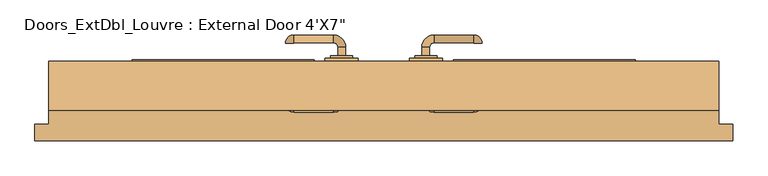
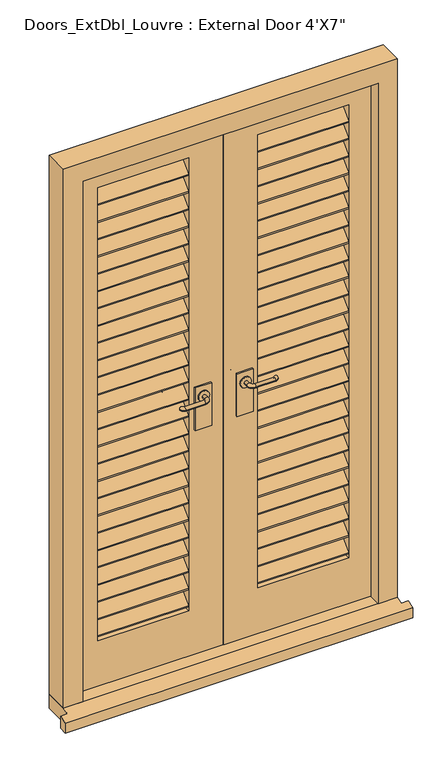
"""IFC4 building model written with IfcOpenShell, lengths in millimetres: door geometry."""

from ifc_helpers import new_model, si_unit, point, frame, frame_2d, origin, place, context, project, spatial, polyline, circle_curve, ellipse_curve, trimmed, segment, composite_curve, outline, extrude, faceted_brep, source, transform, mapped, element, save
from ifc_brep_helpers import plane_surface, cylinder_surface, revolved_surface, advanced_brep


def door_6c7b9bf3(model_context):
    return source(origin(), model_context, "Body", "SolidModel", [
        extrude(outline(polyline([(-0.3, 1896.068), (-0.3, 1900.468), (2.7, 1900.468), (2.7, 1894.8253593), (-41.3, 1850.8253593), (-41.3, 1847.668), (-44.3, 1847.668), (-44.3, 1852.068), (-0.3, 1896.068)])), frame((126.5, 0.0, 0.0), z_axis=(1.0, 0.0, 0.0), x_axis=(0.0, 1.0, 0.0)), (0.0, 0.0, 1.0), 331.6),
        extrude(outline(polyline([(-0.3, 1829.436), (-0.3, 1833.836), (2.7, 1833.836), (2.7, 1828.1933593), (-41.3, 1784.1933593), (-41.3, 1781.036), (-44.3, 1781.036), (-44.3, 1785.436), (-0.3, 1829.436)])), frame((126.5, 0.0, 0.0), z_axis=(1.0, 0.0, 0.0), x_axis=(0.0, 1.0, 0.0)), (0.0, 0.0, 1.0), 331.6),
        extrude(outline(polyline([(-0.3, 1762.804), (-0.3, 1767.204), (2.7, 1767.204), (2.7, 1761.5613593), (-41.3, 1717.5613593), (-41.3, 1714.404), (-44.3, 1714.404), (-44.3, 1718.804), (-0.3, 1762.804)])), frame((126.5, 0.0, 0.0), z_axis=(1.0, 0.0, 0.0), x_axis=(0.0, 1.0, 0.0)), (0.0, 0.0, 1.0), 331.6),
        extrude(outline(polyline([(-0.3, 1696.172), (-0.3, 1700.572), (2.7, 1700.572), (2.7, 1694.9293593), (-41.3, 1650.9293593), (-41.3, 1647.772), (-44.3, 1647.772), (-44.3, 1652.172), (-0.3, 1696.172)])), frame((126.5, 0.0, 0.0), z_axis=(1.0, 0.0, 0.0), x_axis=(0.0, 1.0, 0.0)), (0.0, 0.0, 1.0), 331.6),
        extrude(outline(polyline([(-0.3, 1629.54), (-0.3, 1633.94), (2.7, 1633.94), (2.7, 1628.2973593), (-41.3, 1584.2973593), (-41.3, 1581.14), (-44.3, 1581.14), (-44.3, 1585.54), (-0.3, 1629.54)])), frame((126.5, 0.0, 0.0), z_axis=(1.0, 0.0, 0.0), x_axis=(0.0, 1.0, 0.0)), (0.0, 0.0, 1.0), 331.6),
        extrude(outline(polyline([(-0.3, 1562.908), (-0.3, 1567.308), (2.7, 1567.308), (2.7, 1561.6653593), (-41.3, 1517.6653593), (-41.3, 1514.508), (-44.3, 1514.508), (-44.3, 1518.908), (-0.3, 1562.908)])), frame((126.5, 0.0, 0.0), z_axis=(1.0, 0.0, 0.0), x_axis=(0.0, 1.0, 0.0)), (0.0, 0.0, 1.0), 331.6),
        extrude(outline(polyline([(-0.3, 1496.276), (-0.3, 1500.676), (2.7, 1500.676), (2.7, 1495.0333593), (-41.3, 1451.0333593), (-41.3, 1447.876), (-44.3, 1447.876), (-44.3, 1452.276), (-0.3, 1496.276)])), frame((126.5, 0.0, 0.0), z_axis=(1.0, 0.0, 0.0), x_axis=(0.0, 1.0, 0.0)), (0.0, 0.0, 1.0), 331.6),
        extrude(outline(polyline([(-0.3, 1429.644), (-0.3, 1434.044), (2.7, 1434.044), (2.7, 1428.4013593), (-41.3, 1384.4013593), (-41.3, 1381.244), (-44.3, 1381.244), (-44.3, 1385.644), (-0.3, 1429.644)])), frame((126.5, 0.0, 0.0), z_axis=(1.0, 0.0, 0.0), x_axis=(0.0, 1.0, 0.0)), (0.0, 0.0, 1.0), 331.6),
        extrude(outline(polyline([(-0.3, 1363.012), (-0.3, 1367.412), (2.7, 1367.412), (2.7, 1361.7693593), (-41.3, 1317.7693593), (-41.3, 1314.612), (-44.3, 1314.612), (-44.3, 1319.012), (-0.3, 1363.012)])), frame((126.5, 0.0, 0.0), z_axis=(1.0, 0.0, 0.0), x_axis=(0.0, 1.0, 0.0)), (0.0, 0.0, 1.0), 331.6),
        extrude(outline(polyline([(-0.3, 1296.38), (-0.3, 1300.78), (2.7, 1300.78), (2.7, 1295.1373593), (-41.3, 1251.1373593), (-41.3, 1247.98), (-44.3, 1247.98), (-44.3, 1252.38), (-0.3, 1296.38)])), frame((126.5, 0.0, 0.0), z_axis=(1.0, 0.0, 0.0), x_axis=(0.0, 1.0, 0.0)), (0.0, 0.0, 1.0), 331.6),
        extrude(outline(polyline([(-0.3, 1229.748), (-0.3, 1234.148), (2.7, 1234.148), (2.7, 1228.5053593), (-41.3, 1184.5053593), (-41.3, 1181.348), (-44.3, 1181.348), (-44.3, 1185.748), (-0.3, 1229.748)])), frame((126.5, 0.0, 0.0), z_axis=(1.0, 0.0, 0.0), x_axis=(0.0, 1.0, 0.0)), (0.0, 0.0, 1.0), 331.6),
        extrude(outline(polyline([(-0.3, 1163.116), (-0.3, 1167.516), (2.7, 1167.516), (2.7, 1161.8733593), (-41.3, 1117.8733593), (-41.3, 1114.716), (-44.3, 1114.716), (-44.3, 1119.116), (-0.3, 1163.116)])), frame((126.5, 0.0, 0.0), z_axis=(1.0, 0.0, 0.0), x_axis=(0.0, 1.0, 0.0)), (0.0, 0.0, 1.0), 331.6),
        extrude(outline(polyline([(-0.3, 1096.484), (-0.3, 1100.884), (2.7, 1100.884), (2.7, 1095.2413593), (-41.3, 1051.2413593), (-41.3, 1048.084), (-44.3, 1048.084), (-44.3, 1052.484), (-0.3, 1096.484)])), frame((126.5, 0.0, 0.0), z_axis=(1.0, 0.0, 0.0), x_axis=(0.0, 1.0, 0.0)), (0.0, 0.0, 1.0), 331.6),
        extrude(outline(polyline([(-0.3, 1029.852), (-0.3, 1034.252), (2.7, 1034.252), (2.7, 1028.6093593), (-41.3, 984.6093593), (-41.3, 981.452), (-44.3, 981.452), (-44.3, 985.852), (-0.3, 1029.852)])), frame((126.5, 0.0, 0.0), z_axis=(1.0, 0.0, 0.0), x_axis=(0.0, 1.0, 0.0)), (0.0, 0.0, 1.0), 331.6),
        extrude(outline(polyline([(-0.3, 963.22), (-0.3, 967.62), (2.7, 967.62), (2.7, 961.9773593), (-41.3, 917.9773593), (-41.3, 914.82), (-44.3, 914.82), (-44.3, 919.22), (-0.3, 963.22)])), frame((126.5, 0.0, 0.0), z_axis=(1.0, 0.0, 0.0), x_axis=(0.0, 1.0, 0.0)), (0.0, 0.0, 1.0), 331.6),
        extrude(outline(polyline([(-0.3, 896.588), (-0.3, 900.988), (2.7, 900.988), (2.7, 895.3453593), (-41.3, 851.3453593), (-41.3, 848.188), (-44.3, 848.188), (-44.3, 852.588), (-0.3, 896.588)])), frame((126.5, 0.0, 0.0), z_axis=(1.0, 0.0, 0.0), x_axis=(0.0, 1.0, 0.0)), (0.0, 0.0, 1.0), 331.6),
        extrude(outline(polyline([(-0.3, 829.956), (-0.3, 834.356), (2.7, 834.356), (2.7, 828.7133593), (-41.3, 784.7133593), (-41.3, 781.556), (-44.3, 781.556), (-44.3, 785.956), (-0.3, 829.956)])), frame((126.5, 0.0, 0.0), z_axis=(1.0, 0.0, 0.0), x_axis=(0.0, 1.0, 0.0)), (0.0, 0.0, 1.0), 331.6),
        extrude(outline(polyline([(-0.3, 763.324), (-0.3, 767.724), (2.7, 767.724), (2.7, 762.0813593), (-41.3, 718.0813593), (-41.3, 714.924), (-44.3, 714.924), (-44.3, 719.324), (-0.3, 763.324)])), frame((126.5, 0.0, 0.0), z_axis=(1.0, 0.0, 0.0), x_axis=(0.0, 1.0, 0.0)), (0.0, 0.0, 1.0), 331.6),
        extrude(outline(polyline([(-0.3, 696.692), (-0.3, 701.092), (2.7, 701.092), (2.7, 695.4493593), (-41.3, 651.4493593), (-41.3, 648.292), (-44.3, 648.292), (-44.3, 652.692), (-0.3, 696.692)])), frame((126.5, 0.0, 0.0), z_axis=(1.0, 0.0, 0.0), x_axis=(0.0, 1.0, 0.0)), (0.0, 0.0, 1.0), 331.6),
        extrude(outline(polyline([(-0.3, 630.06), (-0.3, 634.46), (2.7, 634.46), (2.7, 628.8173593), (-41.3, 584.8173593), (-41.3, 581.66), (-44.3, 581.66), (-44.3, 586.06), (-0.3, 630.06)])), frame((126.5, 0.0, 0.0), z_axis=(1.0, 0.0, 0.0), x_axis=(0.0, 1.0, 0.0)), (0.0, 0.0, 1.0), 331.6),
        extrude(outline(polyline([(-0.3, 563.428), (-0.3, 567.828), (2.7, 567.828), (2.7, 562.1853593), (-41.3, 518.1853593), (-41.3, 515.028), (-44.3, 515.028), (-44.3, 519.428), (-0.3, 563.428)])), frame((126.5, 0.0, 0.0), z_axis=(1.0, 0.0, 0.0), x_axis=(0.0, 1.0, 0.0)), (0.0, 0.0, 1.0), 331.6),
        extrude(outline(polyline([(-0.3, 496.796), (-0.3, 501.196), (2.7, 501.196), (2.7, 495.5533593), (-41.3, 451.5533593), (-41.3, 448.396), (-44.3, 448.396), (-44.3, 452.796), (-0.3, 496.796)])), frame((126.5, 0.0, 0.0), z_axis=(1.0, 0.0, 0.0), x_axis=(0.0, 1.0, 0.0)), (0.0, 0.0, 1.0), 331.6),
        extrude(outline(polyline([(-0.3, 430.164), (-0.3, 434.564), (2.7, 434.564), (2.7, 428.9213593), (-41.3, 384.9213593), (-41.3, 381.764), (-44.3, 381.764), (-44.3, 386.164), (-0.3, 430.164)])), frame((126.5, 0.0, 0.0), z_axis=(1.0, 0.0, 0.0), x_axis=(0.0, 1.0, 0.0)), (0.0, 0.0, 1.0), 331.6),
        extrude(outline(polyline([(-0.3, 1896.068), (-0.3, 1900.468), (2.7, 1900.468), (2.7, 1894.8253593), (-41.3, 1850.8253593), (-41.3, 1847.668), (-44.3, 1847.668), (-44.3, 1852.068), (-0.3, 1896.068)])), frame((-458.1, 0.0, 0.0), z_axis=(1.0, 0.0, 0.0), x_axis=(0.0, 1.0, 0.0)), (0.0, 0.0, 1.0), 331.6),
        extrude(outline(polyline([(-0.3, 1829.436), (-0.3, 1833.836), (2.7, 1833.836), (2.7, 1828.1933593), (-41.3, 1784.1933593), (-41.3, 1781.036), (-44.3, 1781.036), (-44.3, 1785.436), (-0.3, 1829.436)])), frame((-458.1, 0.0, 0.0), z_axis=(1.0, 0.0, 0.0), x_axis=(0.0, 1.0, 0.0)), (0.0, 0.0, 1.0), 331.6),
        extrude(outline(polyline([(-0.3, 1762.804), (-0.3, 1767.204), (2.7, 1767.204), (2.7, 1761.5613593), (-41.3, 1717.5613593), (-41.3, 1714.404), (-44.3, 1714.404), (-44.3, 1718.804), (-0.3, 1762.804)])), frame((-458.1, 0.0, 0.0), z_axis=(1.0, 0.0, 0.0), x_axis=(0.0, 1.0, 0.0)), (0.0, 0.0, 1.0), 331.6),
        extrude(outline(polyline([(-0.3, 1696.172), (-0.3, 1700.572), (2.7, 1700.572), (2.7, 1694.9293593), (-41.3, 1650.9293593), (-41.3, 1647.772), (-44.3, 1647.772), (-44.3, 1652.172), (-0.3, 1696.172)])), frame((-458.1, 0.0, 0.0), z_axis=(1.0, 0.0, 0.0), x_axis=(0.0, 1.0, 0.0)), (0.0, 0.0, 1.0), 331.6),
        extrude(outline(polyline([(-0.3, 1629.54), (-0.3, 1633.94), (2.7, 1633.94), (2.7, 1628.2973593), (-41.3, 1584.2973593), (-41.3, 1581.14), (-44.3, 1581.14), (-44.3, 1585.54), (-0.3, 1629.54)])), frame((-458.1, 0.0, 0.0), z_axis=(1.0, 0.0, 0.0), x_axis=(0.0, 1.0, 0.0)), (0.0, 0.0, 1.0), 331.6),
        extrude(outline(polyline([(-0.3, 1562.908), (-0.3, 1567.308), (2.7, 1567.308), (2.7, 1561.6653593), (-41.3, 1517.6653593), (-41.3, 1514.508), (-44.3, 1514.508), (-44.3, 1518.908), (-0.3, 1562.908)])), frame((-458.1, 0.0, 0.0), z_axis=(1.0, 0.0, 0.0), x_axis=(0.0, 1.0, 0.0)), (0.0, 0.0, 1.0), 331.6),
        extrude(outline(polyline([(-0.3, 1496.276), (-0.3, 1500.676), (2.7, 1500.676), (2.7, 1495.0333593), (-41.3, 1451.0333593), (-41.3, 1447.876), (-44.3, 1447.876), (-44.3, 1452.276), (-0.3, 1496.276)])), frame((-458.1, 0.0, 0.0), z_axis=(1.0, 0.0, 0.0), x_axis=(0.0, 1.0, 0.0)), (0.0, 0.0, 1.0), 331.6),
        extrude(outline(polyline([(-0.3, 1429.644), (-0.3, 1434.044), (2.7, 1434.044), (2.7, 1428.4013593), (-41.3, 1384.4013593), (-41.3, 1381.244), (-44.3, 1381.244), (-44.3, 1385.644), (-0.3, 1429.644)])), frame((-458.1, 0.0, 0.0), z_axis=(1.0, 0.0, 0.0), x_axis=(0.0, 1.0, 0.0)), (0.0, 0.0, 1.0), 331.6),
        extrude(outline(polyline([(-0.3, 1363.012), (-0.3, 1367.412), (2.7, 1367.412), (2.7, 1361.7693593), (-41.3, 1317.7693593), (-41.3, 1314.612), (-44.3, 1314.612), (-44.3, 1319.012), (-0.3, 1363.012)])), frame((-458.1, 0.0, 0.0), z_axis=(1.0, 0.0, 0.0), x_axis=(0.0, 1.0, 0.0)), (0.0, 0.0, 1.0), 331.6),
        extrude(outline(polyline([(-0.3, 1296.38), (-0.3, 1300.78), (2.7, 1300.78), (2.7, 1295.1373593), (-41.3, 1251.1373593), (-41.3, 1247.98), (-44.3, 1247.98), (-44.3, 1252.38), (-0.3, 1296.38)])), frame((-458.1, 0.0, 0.0), z_axis=(1.0, 0.0, 0.0), x_axis=(0.0, 1.0, 0.0)), (0.0, 0.0, 1.0), 331.6),
        extrude(outline(polyline([(-0.3, 1229.748), (-0.3, 1234.148), (2.7, 1234.148), (2.7, 1228.5053593), (-41.3, 1184.5053593), (-41.3, 1181.348), (-44.3, 1181.348), (-44.3, 1185.748), (-0.3, 1229.748)])), frame((-458.1, 0.0, 0.0), z_axis=(1.0, 0.0, 0.0), x_axis=(0.0, 1.0, 0.0)), (0.0, 0.0, 1.0), 331.6),
        extrude(outline(polyline([(-0.3, 1163.116), (-0.3, 1167.516), (2.7, 1167.516), (2.7, 1161.8733593), (-41.3, 1117.8733593), (-41.3, 1114.716), (-44.3, 1114.716), (-44.3, 1119.116), (-0.3, 1163.116)])), frame((-458.1, 0.0, 0.0), z_axis=(1.0, 0.0, 0.0), x_axis=(0.0, 1.0, 0.0)), (0.0, 0.0, 1.0), 331.6),
        extrude(outline(polyline([(-0.3, 1096.484), (-0.3, 1100.884), (2.7, 1100.884), (2.7, 1095.2413593), (-41.3, 1051.2413593), (-41.3, 1048.084), (-44.3, 1048.084), (-44.3, 1052.484), (-0.3, 1096.484)])), frame((-458.1, 0.0, 0.0), z_axis=(1.0, 0.0, 0.0), x_axis=(0.0, 1.0, 0.0)), (0.0, 0.0, 1.0), 331.6),
        extrude(outline(polyline([(-0.3, 1029.852), (-0.3, 1034.252), (2.7, 1034.252), (2.7, 1028.6093593), (-41.3, 984.6093593), (-41.3, 981.452), (-44.3, 981.452), (-44.3, 985.852), (-0.3, 1029.852)])), frame((-458.1, 0.0, 0.0), z_axis=(1.0, 0.0, 0.0), x_axis=(0.0, 1.0, 0.0)), (0.0, 0.0, 1.0), 331.6),
        extrude(outline(polyline([(-0.3, 963.22), (-0.3, 967.62), (2.7, 967.62), (2.7, 961.9773593), (-41.3, 917.9773593), (-41.3, 914.82), (-44.3, 914.82), (-44.3, 919.22), (-0.3, 963.22)])), frame((-458.1, 0.0, 0.0), z_axis=(1.0, 0.0, 0.0), x_axis=(0.0, 1.0, 0.0)), (0.0, 0.0, 1.0), 331.6),
        extrude(outline(polyline([(-0.3, 896.588), (-0.3, 900.988), (2.7, 900.988), (2.7, 895.3453593), (-41.3, 851.3453593), (-41.3, 848.188), (-44.3, 848.188), (-44.3, 852.588), (-0.3, 896.588)])), frame((-458.1, 0.0, 0.0), z_axis=(1.0, 0.0, 0.0), x_axis=(0.0, 1.0, 0.0)), (0.0, 0.0, 1.0), 331.6),
        extrude(outline(polyline([(-0.3, 829.956), (-0.3, 834.356), (2.7, 834.356), (2.7, 828.7133593), (-41.3, 784.7133593), (-41.3, 781.556), (-44.3, 781.556), (-44.3, 785.956), (-0.3, 829.956)])), frame((-458.1, 0.0, 0.0), z_axis=(1.0, 0.0, 0.0), x_axis=(0.0, 1.0, 0.0)), (0.0, 0.0, 1.0), 331.6),
        extrude(outline(polyline([(-0.3, 763.324), (-0.3, 767.724), (2.7, 767.724), (2.7, 762.0813593), (-41.3, 718.0813593), (-41.3, 714.924), (-44.3, 714.924), (-44.3, 719.324), (-0.3, 763.324)])), frame((-458.1, 0.0, 0.0), z_axis=(1.0, 0.0, 0.0), x_axis=(0.0, 1.0, 0.0)), (0.0, 0.0, 1.0), 331.6),
        extrude(outline(polyline([(-0.3, 696.692), (-0.3, 701.092), (2.7, 701.092), (2.7, 695.4493593), (-41.3, 651.4493593), (-41.3, 648.292), (-44.3, 648.292), (-44.3, 652.692), (-0.3, 696.692)])), frame((-458.1, 0.0, 0.0), z_axis=(1.0, 0.0, 0.0), x_axis=(0.0, 1.0, 0.0)), (0.0, 0.0, 1.0), 331.6),
        extrude(outline(polyline([(-0.3, 630.06), (-0.3, 634.46), (2.7, 634.46), (2.7, 628.8173593), (-41.3, 584.8173593), (-41.3, 581.66), (-44.3, 581.66), (-44.3, 586.06), (-0.3, 630.06)])), frame((-458.1, 0.0, 0.0), z_axis=(1.0, 0.0, 0.0), x_axis=(0.0, 1.0, 0.0)), (0.0, 0.0, 1.0), 331.6),
        extrude(outline(polyline([(-0.3, 563.428), (-0.3, 567.828), (2.7, 567.828), (2.7, 562.1853593), (-41.3, 518.1853593), (-41.3, 515.028), (-44.3, 515.028), (-44.3, 519.428), (-0.3, 563.428)])), frame((-458.1, 0.0, 0.0), z_axis=(1.0, 0.0, 0.0), x_axis=(0.0, 1.0, 0.0)), (0.0, 0.0, 1.0), 331.6),
        extrude(outline(polyline([(-0.3, 496.796), (-0.3, 501.196), (2.7, 501.196), (2.7, 495.5533593), (-41.3, 451.5533593), (-41.3, 448.396), (-44.3, 448.396), (-44.3, 452.796), (-0.3, 496.796)])), frame((-458.1, 0.0, 0.0), z_axis=(1.0, 0.0, 0.0), x_axis=(0.0, 1.0, 0.0)), (0.0, 0.0, 1.0), 331.6),
        extrude(outline(polyline([(-0.3, 430.164), (-0.3, 434.564), (2.7, 434.564), (2.7, 428.9213593), (-41.3, 384.9213593), (-41.3, 381.764), (-44.3, 381.764), (-44.3, 386.164), (-0.3, 430.164)])), frame((-458.1, 0.0, 0.0), z_axis=(1.0, 0.0, 0.0), x_axis=(0.0, 1.0, 0.0)), (0.0, 0.0, 1.0), 331.6),
        extrude(outline(composite_curve([segment(trimmed(circle_curve(frame_2d((1050.0, 76.5)), 20.0), [point((1050.0, 56.5))], [point((1050.0, 96.5))], False, "CARTESIAN"), True, "CONTINUOUS"), segment(trimmed(circle_curve(frame_2d((1050.0, 76.5)), 20.0), [point((1050.0, 96.5))], [point((1050.0, 56.5))], False, "CARTESIAN"), True, "CONTINUOUS")], self_intersect=False)), frame((0.0, 5.7, 0.0), z_axis=(0.0, 1.0, 0.0), x_axis=(0.0, 0.0, 1.0)), (0.0, 0.0, 1.0), 4.5929895),
        advanced_brep(
        [(83.5, 10.2929895, 1050.0), (69.5, 10.2929895, 1050.0), (83.5, 25.7, 1050.0), (69.5, 25.7, 1050.0), (91.5, 47.7, 1050.0), (91.5, 33.7, 1050.0), (163.5, 33.7, 1050.0), (163.5, 47.7, 1050.0), (164.5, 32.7, 1050.0), (178.5, 32.7, 1050.0)],
        [
            (0, 1, circle_curve(frame((76.5, 10.2929895, 1050.0), z_axis=(0.0, -1.0, 0.0), x_axis=(-1.0, 0.0, 0.0)), 7.0)),
            (1, 0, circle_curve(frame((76.5, 10.2929895, 1050.0), z_axis=(0.0, -1.0, 0.0), x_axis=(-1.0, 0.0, 0.0)), 7.0)),
            (0, 2),
            (2, 3, circle_curve(frame((76.5, 25.7, 1050.0), z_axis=(0.0, -1.0, 0.0), x_axis=(-1.0, 0.0, 0.0)), 7.0)),
            (3, 1),
            (3, 2, circle_curve(frame((76.5, 25.7, 1050.0), z_axis=(0.0, -1.0, 0.0), x_axis=(-1.0, 0.0, 0.0)), 7.0)),
            (4, 3, circle_curve(frame((91.5, 25.7, 1050.0), z_axis=(0.0, 0.0, 1.0), x_axis=(-1.0, 0.0, 0.0)), 22.0)),
            (2, 5, circle_curve(frame((91.5, 25.7, 1050.0), z_axis=(0.0, 0.0, -1.0), x_axis=(-1.0, 0.0, 0.0)), 8.0)),
            (5, 4, circle_curve(frame((91.5, 40.7, 1050.0), z_axis=(-1.0, 0.0, 0.0), x_axis=(0.0, 1.0, 0.0)), 7.0)),
            (4, 5, circle_curve(frame((91.5, 40.7, 1050.0), z_axis=(-1.0, 0.0, 0.0), x_axis=(0.0, 1.0, 0.0)), 7.0)),
            (5, 6),
            (6, 7, circle_curve(frame((163.5, 40.7, 1050.0), z_axis=(-1.0, 0.0, 0.0), x_axis=(0.0, 1.0, 0.0)), 7.0)),
            (7, 4),
            (7, 6, circle_curve(frame((163.5, 40.7, 1050.0), z_axis=(-1.0, 0.0, 0.0), x_axis=(0.0, 1.0, 0.0)), 7.0)),
            (8, 9, circle_curve(frame((171.5, 32.7, 1050.0), z_axis=(0.0, -1.0, 0.0), x_axis=(1.0, 0.0, 0.0)), 7.0)),
            (9, 8, circle_curve(frame((171.5, 32.7, 1050.0), z_axis=(0.0, -1.0, 0.0), x_axis=(1.0, 0.0, 0.0)), 7.0)),
            (9, 7, circle_curve(frame((163.5, 32.7, 1050.0), z_axis=(0.0, 0.0, 1.0), x_axis=(0.0, 1.0, 0.0)), 15.0)),
            (6, 8, circle_curve(frame((163.5, 32.7, 1050.0), z_axis=(0.0, 0.0, -1.0), x_axis=(0.0, 1.0, 0.0)), 1.0)),
        ],
        [
            plane_surface(frame((76.5, 10.2929895, 1050.0), z_axis=(0.0, -1.0, 0.0), x_axis=(0.0, 0.0, 1.0))),
            cylinder_surface(frame((76.5, 10.2929895, 1050.0), z_axis=(0.0, -1.0, 0.0), x_axis=(-1.0, 0.0, 0.0)), 7.0),
            revolved_surface(trimmed(ellipse_curve(frame((76.5, 25.7, 1050.0), z_axis=(0.0, -1.0, 0.0), x_axis=(-1.0, 0.0, 0.0)), 7.0, 7.0), [point((83.5, 25.7, 1050.0))], [point((69.5, 25.7, 1050.0))], True, "CARTESIAN"), (91.5, 25.7, 1050.0), (0.0, 0.0, -1.0)),
            revolved_surface(trimmed(ellipse_curve(frame((76.5, 25.7, 1050.0), z_axis=(0.0, -1.0, 0.0), x_axis=(-1.0, 0.0, 0.0)), 7.0, 7.0), [point((69.5, 25.7, 1050.0))], [point((83.5, 25.7, 1050.0))], True, "CARTESIAN"), (91.5, 25.7, 1050.0), (0.0, 0.0, -1.0)),
            cylinder_surface(frame((91.5, 40.7, 1050.0), z_axis=(-1.0, 0.0, 0.0), x_axis=(0.0, 1.0, 0.0)), 7.0),
            plane_surface(frame((171.5, 32.7, 1050.0), z_axis=(0.0, -1.0, 0.0), x_axis=(0.0, 0.0, 1.0))),
            revolved_surface(trimmed(ellipse_curve(frame((163.5, 40.7, 1050.0), z_axis=(-1.0, 0.0, 0.0), x_axis=(0.0, 1.0, 0.0)), 7.0, 7.0), [point((163.5, 33.7, 1050.0))], [point((163.5, 47.7, 1050.0))], True, "CARTESIAN"), (163.5, 32.7, 1050.0), (0.0, 0.0, -1.0)),
            revolved_surface(trimmed(ellipse_curve(frame((163.5, 40.7, 1050.0), z_axis=(-1.0, 0.0, 0.0), x_axis=(0.0, 1.0, 0.0)), 7.0, 7.0), [point((163.5, 47.7, 1050.0))], [point((163.5, 33.7, 1050.0))], True, "CARTESIAN"), (163.5, 32.7, 1050.0), (0.0, 0.0, -1.0)),
        ],
        [
            (0, [[1, 2]]),
            (1, [[-1, 3, 4, 5]]),
            (1, [[-2, -5, 6, -3]]),
            (2, [[7, -4, 8, 9]]),
            (3, [[-8, -6, -7, 10]]),
            (4, [[-9, 11, 12, 13]]),
            (4, [[-10, -13, 14, -11]]),
            (5, [[15, 16]]),
            (6, [[17, -12, 18, -16]]),
            (7, [[-18, -14, -17, -15]]),
        ],
    ),
        extrude(outline(polyline([(106.5, -0.3), (46.5, -0.3), (46.5, 5.7), (106.5, 5.7), (106.5, -0.3)])), frame((0.0, 0.0, 925.0), z_axis=(0.0, 0.0, 1.0), x_axis=(1.0, 0.0, 0.0)), (0.0, 0.0, 1.0), 165.0),
        extrude(outline(composite_curve([segment(trimmed(circle_curve(frame_2d((1050.0, -76.5)), 20.0), [point((1050.0, -56.5))], [point((1050.0, -96.5))], False, "CARTESIAN"), True, "CONTINUOUS"), segment(trimmed(circle_curve(frame_2d((1050.0, -76.5)), 20.0), [point((1050.0, -96.5))], [point((1050.0, -56.5))], False, "CARTESIAN"), True, "CONTINUOUS")], self_intersect=False)), frame((0.0, 5.7, 0.0), z_axis=(0.0, 1.0, 0.0), x_axis=(0.0, 0.0, 1.0)), (0.0, 0.0, 1.0), 4.5929895),
        advanced_brep(
        [(-83.5, 10.2929895, 1050.0), (-69.5, 10.2929895, 1050.0), (-69.5, 25.7, 1050.0), (-83.5, 25.7, 1050.0), (-91.5, 47.7, 1050.0), (-91.5, 33.7, 1050.0), (-163.5, 47.7, 1050.0), (-163.5, 33.7, 1050.0), (-164.5, 32.7, 1050.0), (-178.5, 32.7, 1050.0)],
        [
            (0, 1, circle_curve(frame((-76.5, 10.2929895, 1050.0), z_axis=(0.0, -1.0, 0.0), x_axis=(1.0, 0.0, 0.0)), 7.0)),
            (1, 0, circle_curve(frame((-76.5, 10.2929895, 1050.0), z_axis=(0.0, -1.0, 0.0), x_axis=(1.0, 0.0, 0.0)), 7.0)),
            (1, 2),
            (2, 3, circle_curve(frame((-76.5, 25.7, 1050.0), z_axis=(0.0, -1.0, 0.0), x_axis=(1.0, 0.0, 0.0)), 7.0)),
            (3, 0),
            (3, 2, circle_curve(frame((-76.5, 25.7, 1050.0), z_axis=(0.0, -1.0, 0.0), x_axis=(1.0, 0.0, 0.0)), 7.0)),
            (4, 5, circle_curve(frame((-91.5, 40.7, 1050.0), z_axis=(1.0, 0.0, 0.0), x_axis=(0.0, 1.0, 0.0)), 7.0)),
            (5, 3, circle_curve(frame((-91.5, 25.7, 1050.0), z_axis=(0.0, 0.0, -1.0), x_axis=(1.0, 0.0, 0.0)), 8.0)),
            (2, 4, circle_curve(frame((-91.5, 25.7, 1050.0), z_axis=(0.0, 0.0, 1.0), x_axis=(1.0, 0.0, 0.0)), 22.0)),
            (5, 4, circle_curve(frame((-91.5, 40.7, 1050.0), z_axis=(1.0, 0.0, 0.0), x_axis=(0.0, 1.0, 0.0)), 7.0)),
            (4, 6),
            (6, 7, circle_curve(frame((-163.5, 40.7, 1050.0), z_axis=(1.0, 0.0, 0.0), x_axis=(0.0, 1.0, 0.0)), 7.0)),
            (7, 5),
            (7, 6, circle_curve(frame((-163.5, 40.7, 1050.0), z_axis=(1.0, 0.0, 0.0), x_axis=(0.0, 1.0, 0.0)), 7.0)),
            (8, 9, circle_curve(frame((-171.5, 32.7, 1050.0), z_axis=(0.0, -1.0, 0.0), x_axis=(-1.0, 0.0, 0.0)), 7.0)),
            (9, 8, circle_curve(frame((-171.5, 32.7, 1050.0), z_axis=(0.0, -1.0, 0.0), x_axis=(-1.0, 0.0, 0.0)), 7.0)),
            (8, 7, circle_curve(frame((-163.5, 32.7, 1050.0), z_axis=(0.0, 0.0, -1.0), x_axis=(0.0, 1.0, 0.0)), 1.0)),
            (6, 9, circle_curve(frame((-163.5, 32.7, 1050.0), z_axis=(0.0, 0.0, 1.0), x_axis=(0.0, 1.0, 0.0)), 15.0)),
        ],
        [
            plane_surface(frame((-76.5, 10.2929895, 1050.0), z_axis=(0.0, -1.0, 0.0), x_axis=(0.0, 0.0, 1.0))),
            cylinder_surface(frame((-76.5, 10.2929895, 1050.0), z_axis=(0.0, -1.0, 0.0), x_axis=(1.0, 0.0, 0.0)), 7.0),
            revolved_surface(trimmed(ellipse_curve(frame((-76.5, 25.7, 1050.0), z_axis=(0.0, 1.0, 0.0), x_axis=(1.0, 0.0, 0.0)), 7.0, 7.0), [point((-83.5, 25.7, 1050.0))], [point((-69.5, 25.7, 1050.0))], True, "CARTESIAN"), (-91.5, 25.7, 1050.0), (0.0, 0.0, -1.0)),
            revolved_surface(trimmed(ellipse_curve(frame((-76.5, 25.7, 1050.0), z_axis=(0.0, 1.0, 0.0), x_axis=(1.0, 0.0, 0.0)), 7.0, 7.0), [point((-69.5, 25.7, 1050.0))], [point((-83.5, 25.7, 1050.0))], True, "CARTESIAN"), (-91.5, 25.7, 1050.0), (0.0, 0.0, -1.0)),
            cylinder_surface(frame((-91.5, 40.7, 1050.0), z_axis=(1.0, 0.0, 0.0), x_axis=(0.0, 1.0, 0.0)), 7.0),
            plane_surface(frame((-171.5, 32.7, 1050.0), z_axis=(0.0, -1.0, 0.0), x_axis=(0.0, 0.0, 1.0))),
            revolved_surface(trimmed(ellipse_curve(frame((-163.5, 40.7, 1050.0), z_axis=(-1.0, 0.0, 0.0), x_axis=(0.0, 1.0, 0.0)), 7.0, 7.0), [point((-163.5, 33.7, 1050.0))], [point((-163.5, 47.7, 1050.0))], True, "CARTESIAN"), (-163.5, 32.7, 1050.0), (0.0, 0.0, -1.0)),
            revolved_surface(trimmed(ellipse_curve(frame((-163.5, 40.7, 1050.0), z_axis=(-1.0, 0.0, 0.0), x_axis=(0.0, 1.0, 0.0)), 7.0, 7.0), [point((-163.5, 47.7, 1050.0))], [point((-163.5, 33.7, 1050.0))], True, "CARTESIAN"), (-163.5, 32.7, 1050.0), (0.0, 0.0, -1.0)),
        ],
        [
            (0, [[1, 2]]),
            (1, [[3, 4, 5, -2]]),
            (1, [[-5, 6, -3, -1]]),
            (2, [[7, 8, -4, 9]]),
            (3, [[10, -9, -6, -8]]),
            (4, [[11, 12, 13, -7]]),
            (4, [[-13, 14, -11, -10]]),
            (5, [[15, 16]]),
            (6, [[-15, 17, -12, 18]]),
            (7, [[-16, -18, -14, -17]]),
        ],
    ),
        extrude(outline(polyline([(-106.5, -0.3), (-106.5, 5.7), (-46.5, 5.7), (-46.5, -0.3), (-106.5, -0.3)])), frame((0.0, 0.0, 925.0), z_axis=(0.0, 0.0, 1.0), x_axis=(1.0, 0.0, 0.0)), (0.0, 0.0, 1.0), 165.0),
        extrude(outline(composite_curve([segment(trimmed(circle_curve(frame_2d((1050.0, -76.5)), 20.0), [point((1050.0, -56.5))], [point((1050.0, -96.5))], False, "CARTESIAN"), True, "CONTINUOUS"), segment(trimmed(circle_curve(frame_2d((1050.0, -76.5)), 20.0), [point((1050.0, -96.5))], [point((1050.0, -56.5))], False, "CARTESIAN"), True, "CONTINUOUS")], self_intersect=False)), frame((0.0, -54.8929895, 0.0), z_axis=(0.0, 1.0, 0.0), x_axis=(0.0, 0.0, 1.0)), (0.0, 0.0, 1.0), 4.5929895),
        advanced_brep(
        [(-83.5, -54.8929895, 1050.0), (-69.5, -54.8929895, 1050.0), (-83.5, -70.3, 1050.0), (-69.5, -70.3, 1050.0), (-91.5, -92.3, 1050.0), (-91.5, -78.3, 1050.0), (-163.5, -78.3, 1050.0), (-163.5, -92.3, 1050.0), (-164.5, -77.3, 1050.0), (-178.5, -77.3, 1050.0)],
        [
            (0, 1, circle_curve(frame((-76.5, -54.8929895, 1050.0), z_axis=(0.0, 1.0, 0.0), x_axis=(1.0, 0.0, 0.0)), 7.0)),
            (1, 0, circle_curve(frame((-76.5, -54.8929895, 1050.0), z_axis=(0.0, 1.0, 0.0), x_axis=(1.0, 0.0, 0.0)), 7.0)),
            (0, 2),
            (2, 3, circle_curve(frame((-76.5, -70.3, 1050.0), z_axis=(0.0, 1.0, 0.0), x_axis=(1.0, 0.0, 0.0)), 7.0)),
            (3, 1),
            (3, 2, circle_curve(frame((-76.5, -70.3, 1050.0), z_axis=(0.0, 1.0, 0.0), x_axis=(1.0, 0.0, 0.0)), 7.0)),
            (4, 3, circle_curve(frame((-91.5, -70.3, 1050.0), z_axis=(0.0, 0.0, 1.0), x_axis=(1.0, 0.0, 0.0)), 22.0)),
            (2, 5, circle_curve(frame((-91.5, -70.3, 1050.0), z_axis=(0.0, 0.0, -1.0), x_axis=(1.0, 0.0, 0.0)), 8.0)),
            (5, 4, circle_curve(frame((-91.5, -85.3, 1050.0), z_axis=(1.0, 0.0, 0.0), x_axis=(0.0, -1.0, 0.0)), 7.0)),
            (4, 5, circle_curve(frame((-91.5, -85.3, 1050.0), z_axis=(1.0, 0.0, 0.0), x_axis=(0.0, -1.0, 0.0)), 7.0)),
            (5, 6),
            (6, 7, circle_curve(frame((-163.5, -85.3, 1050.0), z_axis=(1.0, 0.0, 0.0), x_axis=(0.0, -1.0, 0.0)), 7.0)),
            (7, 4),
            (7, 6, circle_curve(frame((-163.5, -85.3, 1050.0), z_axis=(1.0, 0.0, 0.0), x_axis=(0.0, -1.0, 0.0)), 7.0)),
            (8, 9, circle_curve(frame((-171.5, -77.3, 1050.0), z_axis=(0.0, 1.0, 0.0), x_axis=(-1.0, 0.0, 0.0)), 7.0)),
            (9, 8, circle_curve(frame((-171.5, -77.3, 1050.0), z_axis=(0.0, 1.0, 0.0), x_axis=(-1.0, 0.0, 0.0)), 7.0)),
            (9, 7, circle_curve(frame((-163.5, -77.3, 1050.0), z_axis=(0.0, 0.0, 1.0), x_axis=(0.0, -1.0, 0.0)), 15.0)),
            (6, 8, circle_curve(frame((-163.5, -77.3, 1050.0), z_axis=(0.0, 0.0, -1.0), x_axis=(0.0, -1.0, 0.0)), 1.0)),
        ],
        [
            plane_surface(frame((-76.5, -54.8929895, 1050.0), z_axis=(0.0, 1.0, 0.0), x_axis=(0.0, 0.0, 1.0))),
            cylinder_surface(frame((-76.5, -54.8929895, 1050.0), z_axis=(0.0, 1.0, 0.0), x_axis=(1.0, 0.0, 0.0)), 7.0),
            revolved_surface(trimmed(ellipse_curve(frame((-76.5, -70.3, 1050.0), z_axis=(0.0, 1.0, 0.0), x_axis=(1.0, 0.0, 0.0)), 7.0, 7.0), [point((-83.5, -70.3, 1050.0))], [point((-69.5, -70.3, 1050.0))], True, "CARTESIAN"), (-91.5, -70.3, 1050.0), (0.0, 0.0, -1.0)),
            revolved_surface(trimmed(ellipse_curve(frame((-76.5, -70.3, 1050.0), z_axis=(0.0, 1.0, 0.0), x_axis=(1.0, 0.0, 0.0)), 7.0, 7.0), [point((-69.5, -70.3, 1050.0))], [point((-83.5, -70.3, 1050.0))], True, "CARTESIAN"), (-91.5, -70.3, 1050.0), (0.0, 0.0, -1.0)),
            cylinder_surface(frame((-91.5, -85.3, 1050.0), z_axis=(1.0, 0.0, 0.0), x_axis=(0.0, -1.0, 0.0)), 7.0),
            plane_surface(frame((-171.5, -77.3, 1050.0), z_axis=(0.0, 1.0, 0.0), x_axis=(0.0, 0.0, 1.0))),
            revolved_surface(trimmed(ellipse_curve(frame((-163.5, -85.3, 1050.0), z_axis=(1.0, 0.0, 0.0), x_axis=(0.0, -1.0, 0.0)), 7.0, 7.0), [point((-163.5, -78.3, 1050.0))], [point((-163.5, -92.3, 1050.0))], True, "CARTESIAN"), (-163.5, -77.3, 1050.0), (0.0, 0.0, -1.0)),
            revolved_surface(trimmed(ellipse_curve(frame((-163.5, -85.3, 1050.0), z_axis=(1.0, 0.0, 0.0), x_axis=(0.0, -1.0, 0.0)), 7.0, 7.0), [point((-163.5, -92.3, 1050.0))], [point((-163.5, -78.3, 1050.0))], True, "CARTESIAN"), (-163.5, -77.3, 1050.0), (0.0, 0.0, -1.0)),
        ],
        [
            (0, [[1, 2]]),
            (1, [[-1, 3, 4, 5]]),
            (1, [[-2, -5, 6, -3]]),
            (2, [[7, -4, 8, 9]]),
            (3, [[-8, -6, -7, 10]]),
            (4, [[-9, 11, 12, 13]]),
            (4, [[-10, -13, 14, -11]]),
            (5, [[15, 16]]),
            (6, [[17, -12, 18, -16]]),
            (7, [[-18, -14, -17, -15]]),
        ],
    ),
        extrude(outline(polyline([(-106.5, -44.3), (-46.5, -44.3), (-46.5, -50.3), (-106.5, -50.3), (-106.5, -44.3)])), frame((0.0, 0.0, 925.0), z_axis=(0.0, 0.0, 1.0), x_axis=(1.0, 0.0, 0.0)), (0.0, 0.0, 1.0), 165.0),
        extrude(outline(composite_curve([segment(trimmed(circle_curve(frame_2d((1050.0, 76.5)), 20.0), [point((1050.0, 56.5))], [point((1050.0, 96.5))], False, "CARTESIAN"), True, "CONTINUOUS"), segment(trimmed(circle_curve(frame_2d((1050.0, 76.5)), 20.0), [point((1050.0, 96.5))], [point((1050.0, 56.5))], False, "CARTESIAN"), True, "CONTINUOUS")], self_intersect=False)), frame((0.0, -54.8929895, 0.0), z_axis=(0.0, 1.0, 0.0), x_axis=(0.0, 0.0, 1.0)), (0.0, 0.0, 1.0), 4.5929895),
        advanced_brep(
        [(83.5, -54.8929895, 1050.0), (69.5, -54.8929895, 1050.0), (69.5, -70.3, 1050.0), (83.5, -70.3, 1050.0), (91.5, -92.3, 1050.0), (91.5, -78.3, 1050.0), (163.5, -92.3, 1050.0), (163.5, -78.3, 1050.0), (164.5, -77.3, 1050.0), (178.5, -77.3, 1050.0)],
        [
            (0, 1, circle_curve(frame((76.5, -54.8929895, 1050.0), z_axis=(0.0, 1.0, 0.0), x_axis=(-1.0, 0.0, 0.0)), 7.0)),
            (1, 0, circle_curve(frame((76.5, -54.8929895, 1050.0), z_axis=(0.0, 1.0, 0.0), x_axis=(-1.0, 0.0, 0.0)), 7.0)),
            (1, 2),
            (2, 3, circle_curve(frame((76.5, -70.3, 1050.0), z_axis=(0.0, 1.0, 0.0), x_axis=(-1.0, 0.0, 0.0)), 7.0)),
            (3, 0),
            (3, 2, circle_curve(frame((76.5, -70.3, 1050.0), z_axis=(0.0, 1.0, 0.0), x_axis=(-1.0, 0.0, 0.0)), 7.0)),
            (4, 5, circle_curve(frame((91.5, -85.3, 1050.0), z_axis=(-1.0, 0.0, 0.0), x_axis=(0.0, -1.0, 0.0)), 7.0)),
            (5, 3, circle_curve(frame((91.5, -70.3, 1050.0), z_axis=(0.0, 0.0, -1.0), x_axis=(-1.0, 0.0, 0.0)), 8.0)),
            (2, 4, circle_curve(frame((91.5, -70.3, 1050.0), z_axis=(0.0, 0.0, 1.0), x_axis=(-1.0, 0.0, 0.0)), 22.0)),
            (5, 4, circle_curve(frame((91.5, -85.3, 1050.0), z_axis=(-1.0, 0.0, 0.0), x_axis=(0.0, -1.0, 0.0)), 7.0)),
            (4, 6),
            (6, 7, circle_curve(frame((163.5, -85.3, 1050.0), z_axis=(-1.0, 0.0, 0.0), x_axis=(0.0, -1.0, 0.0)), 7.0)),
            (7, 5),
            (7, 6, circle_curve(frame((163.5, -85.3, 1050.0), z_axis=(-1.0, 0.0, 0.0), x_axis=(0.0, -1.0, 0.0)), 7.0)),
            (8, 9, circle_curve(frame((171.5, -77.3, 1050.0), z_axis=(0.0, 1.0, 0.0), x_axis=(1.0, 0.0, 0.0)), 7.0)),
            (9, 8, circle_curve(frame((171.5, -77.3, 1050.0), z_axis=(0.0, 1.0, 0.0), x_axis=(1.0, 0.0, 0.0)), 7.0)),
            (8, 7, circle_curve(frame((163.5, -77.3, 1050.0), z_axis=(0.0, 0.0, -1.0), x_axis=(0.0, -1.0, 0.0)), 1.0)),
            (6, 9, circle_curve(frame((163.5, -77.3, 1050.0), z_axis=(0.0, 0.0, 1.0), x_axis=(0.0, -1.0, 0.0)), 15.0)),
        ],
        [
            plane_surface(frame((76.5, -54.8929895, 1050.0), z_axis=(0.0, 1.0, 0.0), x_axis=(0.0, 0.0, 1.0))),
            cylinder_surface(frame((76.5, -54.8929895, 1050.0), z_axis=(0.0, 1.0, 0.0), x_axis=(-1.0, 0.0, 0.0)), 7.0),
            revolved_surface(trimmed(ellipse_curve(frame((76.5, -70.3, 1050.0), z_axis=(0.0, -1.0, 0.0), x_axis=(-1.0, 0.0, 0.0)), 7.0, 7.0), [point((83.5, -70.3, 1050.0))], [point((69.5, -70.3, 1050.0))], True, "CARTESIAN"), (91.5, -70.3, 1050.0), (0.0, 0.0, -1.0)),
            revolved_surface(trimmed(ellipse_curve(frame((76.5, -70.3, 1050.0), z_axis=(0.0, -1.0, 0.0), x_axis=(-1.0, 0.0, 0.0)), 7.0, 7.0), [point((69.5, -70.3, 1050.0))], [point((83.5, -70.3, 1050.0))], True, "CARTESIAN"), (91.5, -70.3, 1050.0), (0.0, 0.0, -1.0)),
            cylinder_surface(frame((91.5, -85.3, 1050.0), z_axis=(-1.0, 0.0, 0.0), x_axis=(0.0, -1.0, 0.0)), 7.0),
            plane_surface(frame((171.5, -77.3, 1050.0), z_axis=(0.0, 1.0, 0.0), x_axis=(0.0, 0.0, 1.0))),
            revolved_surface(trimmed(ellipse_curve(frame((163.5, -85.3, 1050.0), z_axis=(1.0, 0.0, 0.0), x_axis=(0.0, -1.0, 0.0)), 7.0, 7.0), [point((163.5, -78.3, 1050.0))], [point((163.5, -92.3, 1050.0))], True, "CARTESIAN"), (163.5, -77.3, 1050.0), (0.0, 0.0, -1.0)),
            revolved_surface(trimmed(ellipse_curve(frame((163.5, -85.3, 1050.0), z_axis=(1.0, 0.0, 0.0), x_axis=(0.0, -1.0, 0.0)), 7.0, 7.0), [point((163.5, -92.3, 1050.0))], [point((163.5, -78.3, 1050.0))], True, "CARTESIAN"), (163.5, -77.3, 1050.0), (0.0, 0.0, -1.0)),
        ],
        [
            (0, [[1, 2]]),
            (1, [[3, 4, 5, -2]]),
            (1, [[-5, 6, -3, -1]]),
            (2, [[7, 8, -4, 9]]),
            (3, [[10, -9, -6, -8]]),
            (4, [[11, 12, 13, -7]]),
            (4, [[-13, 14, -11, -10]]),
            (5, [[15, 16]]),
            (6, [[-15, 17, -12, 18]]),
            (7, [[-16, -18, -14, -17]]),
        ],
    ),
        extrude(outline(polyline([(106.5, -44.3), (106.5, -50.3), (46.5, -50.3), (46.5, -44.3), (106.5, -44.3)])), frame((0.0, 0.0, 925.0), z_axis=(0.0, 0.0, 1.0), x_axis=(1.0, 0.0, 0.0)), (0.0, 0.0, 1.0), 165.0),
        extrude(outline(polyline([(-0.3, 363.532), (-0.3, 367.932), (2.7, 367.932), (2.7, 362.2893593), (-41.3, 318.2893593), (-41.3, 315.132), (-44.3, 315.132), (-44.3, 319.532), (-0.3, 363.532)])), frame((126.5, 0.0, 0.0), z_axis=(1.0, 0.0, 0.0), x_axis=(0.0, 1.0, 0.0)), (0.0, 0.0, 1.0), 331.6),
        extrude(outline(polyline([(-0.3, 363.532), (-0.3, 367.932), (2.7, 367.932), (2.7, 362.2893593), (-41.3, 318.2893593), (-41.3, 315.132), (-44.3, 315.132), (-44.3, 319.532), (-0.3, 363.532)])), frame((-458.1, 0.0, 0.0), z_axis=(1.0, 0.0, 0.0), x_axis=(0.0, 1.0, 0.0)), (0.0, 0.0, 1.0), 331.6),
        extrude(outline(polyline([(-0.3, 1962.7), (-0.3, 1967.1), (2.7, 1967.1), (2.7, 1961.4573593), (-41.3, 1917.4573593), (-41.3, 1914.3), (-44.3, 1914.3), (-44.3, 1918.7), (-0.3, 1962.7)])), frame((126.5, 0.0, 0.0), z_axis=(1.0, 0.0, 0.0), x_axis=(0.0, 1.0, 0.0)), (0.0, 0.0, 1.0), 331.6),
        extrude(outline(polyline([(-0.3, 296.9), (-0.3, 301.3), (2.7, 301.3), (2.7, 295.6573593), (-41.3, 251.6573593), (-41.3, 248.5), (-44.3, 248.5), (-44.3, 252.9), (-0.3, 296.9)])), frame((126.5, 0.0, 0.0), z_axis=(1.0, 0.0, 0.0), x_axis=(0.0, 1.0, 0.0)), (0.0, 0.0, 1.0), 331.6),
        extrude(outline(polyline([(-0.3, 1962.7), (-0.3, 1967.1), (2.7, 1967.1), (2.7, 1961.4573593), (-41.3, 1917.4573593), (-41.3, 1914.3), (-44.3, 1914.3), (-44.3, 1918.7), (-0.3, 1962.7)])), frame((-458.1, 0.0, 0.0), z_axis=(1.0, 0.0, 0.0), x_axis=(0.0, 1.0, 0.0)), (0.0, 0.0, 1.0), 331.6),
        extrude(outline(polyline([(-0.3, 296.9), (-0.3, 301.3), (2.7, 301.3), (2.7, 295.6573593), (-41.3, 251.6573593), (-41.3, 248.5), (-44.3, 248.5), (-44.3, 252.9), (-0.3, 296.9)])), frame((-458.1, 0.0, 0.0), z_axis=(1.0, 0.0, 0.0), x_axis=(0.0, 1.0, 0.0)), (0.0, 0.0, 1.0), 331.6),
        faceted_brep([(539.1, -89.3, 54.5), (539.1, -47.3, 54.5), (561.1, -47.3, 54.5), (561.1, -0.3, 54.5), (609.6, -0.3, 54.5), (609.6, -89.3, 54.5), (609.6, -89.3, 2133.6), (-609.6, -89.3, 2133.6), (-609.6, -89.3, 54.5), (-539.1, -89.3, 54.5), (-539.1, -89.3, 2063.1), (539.1, -89.3, 2063.1), (609.6, -0.3, 2133.6), (561.1, -0.3, 2085.1), (-561.1, -0.3, 2085.1), (-561.1, -0.3, 54.5), (-609.6, -0.3, 54.5), (-609.6, -0.3, 2133.6), (561.1, -47.3, 2085.1), (539.1, -47.3, 2063.1), (-539.1, -47.3, 2063.1), (-539.1, -47.3, 54.5), (-561.1, -47.3, 54.5), (-561.1, -47.3, 2085.1)], [[[0, 1, 2, 3, 4, 5]], [[5, 6, 7, 8, 9, 10, 11, 0]], [[4, 12, 6, 5]], [[3, 13, 14, 15, 16, 17, 12, 4]], [[2, 18, 13, 3]], [[1, 19, 20, 21, 22, 23, 18, 2]], [[0, 11, 19, 1]], [[10, 9, 21, 20]], [[9, 8, 16, 15, 22, 21]], [[17, 16, 8, 7]], [[23, 22, 15, 14]], [[12, 17, 7, 6]], [[18, 23, 14, 13]], [[11, 10, 20, 19]]]),
        extrude(outline(polyline([(58.5, 558.1), (2082.1, 558.1), (2082.1, 1.5), (58.5, 1.5), (58.5, 558.1)]), holes=[polyline([(1982.1, 458.1), (233.5, 458.1), (233.5, 126.5), (1982.1, 126.5), (1982.1, 458.1)])]), frame((0.0, -44.3, 0.0), z_axis=(0.0, 1.0, 0.0), x_axis=(0.0, 0.0, 1.0)), (0.0, 0.0, 1.0), 44.0),
        extrude(outline(polyline([(58.5, -558.1), (58.5, -1.5), (2082.1, -1.5), (2082.1, -558.1), (58.5, -558.1)]), holes=[polyline([(1982.1, -126.5), (233.5, -126.5), (233.5, -458.1), (1982.1, -458.1), (1982.1, -126.5)])]), frame((0.0, -44.3, 0.0), z_axis=(0.0, 1.0, 0.0), x_axis=(0.0, 0.0, 1.0)), (0.0, 0.0, 1.0), 44.0),
        faceted_brep([(634.6, -144.3, 0.0), (634.6, -114.3, 0.0), (634.6, -114.3, 47.2703282), (634.6, -144.3, 38.5947221), (-634.6, -144.3, 38.5947221), (-634.6, -114.3, 47.2703282), (-634.6, -114.3, 0.0), (-634.6, -144.3, 0.0), (-609.6, -114.3, 0.0), (-609.6, -0.3, 0.0), (609.6, -0.3, 0.0), (609.6, -114.3, 0.0), (609.6, -114.3, 47.2703282), (609.6, -89.3, 54.5), (-609.6, -89.3, 54.5), (-609.6, -114.3, 47.2703282), (609.6, -0.3, 54.5), (-609.6, -0.3, 54.5)], [[[0, 1, 2, 3]], [[4, 5, 6, 7]], [[7, 6, 8, 9, 10, 11, 1, 0]], [[3, 4, 7, 0]], [[3, 2, 12, 13, 14, 15, 5, 4]], [[14, 13, 16, 17]], [[17, 16, 10, 9]], [[15, 14, 17, 9, 8]], [[8, 6, 5, 15]], [[11, 10, 16, 13, 12]], [[12, 2, 1, 11]]]),
    ])


if __name__ == "__main__":
    model = new_model("IFC4")
    model_context = context("Model", 3, world=origin())
    ifc_project = project(units=[si_unit("LENGTHUNIT", "METRE", prefix="MILLI")], contexts=[model_context])
    site = spatial("IfcSite", under=ifc_project)
    building = spatial("IfcBuilding", under=site)
    placement = place(None, origin())
    door_shape = door_6c7b9bf3(model_context)
    element("IfcDoor", 1, ObjectType="Doors_ExtDbl_Louvre : External Door 4'X7\"", at=placement, inside=building, context=model_context, shape_type="MappedRepresentation", body=[
        mapped(door_shape, transform((0.0, 0.0, 0.0), x_axis=(1.0, 0.0, 0.0), y_axis=(0.0, 1.0, 0.0), z_axis=(0.0, 0.0, 1.0))),
    ])
    save(model, "model.ifc")

# Revit data of these elements
# Type "Doors_ExtDbl_Louvre : External Door 4'X7\""
#   Type Mark = "10"
#   Type Comments = "External Double"
#   Operation = "DoubleDoorSingleSwing"
#   Construction Type Id = "MDOOR"
#   Keynote = "L20"
#   Analytic Construction = "Metal"
#   Wrap Layers (Int) from Ext = 0' - 6.98819"
#   Wrap Layers (Ext) from Ext = 0' - 4.03543"
#   Thickness = 0' - 1.73228"
#   Stile Top Rail = 0' - 3.93701"
#   Stile Shutting = 0' - 4.92126"
#   Stile Hanging = 0' - 3.93701"
#   Stile Bottom Rail = 0' - 6.88976"
#   Rough Width = 4' - 0"
#   Rough Height = 7' - 0"
#   O/A Frame Width = 0' - 2.51969"
#   Heat Transfer Coefficient (U) = 0.651978 BTU/(h·ft²·°F)
#   Handle Z Distance = 3' - 5.33858"
#   FrameWidth = 0' - 1.65354"
#   FrameOffset - External = 0' - 0.98425"
#   FrameDepth = 0' - 3.50394"
#   Door Panel Width = 1' - 9.91339"
#   Door Panel Thickness = 0' - 1.73228"
#   Door Panel Height = 6' - 7.66929"
#   DONT CHANGE Louvre Length = 1' - 1.05512"
#   Cill Thickness = 0' - 2.14567"
#   Cill Projection = 0' - 1.1811"
#   Handle X Distance = 0' - 2.95276"
#   Height = 7' - 0"
#   Structural Tolerance = 0' - 0.25591"
#   Tolerance = 0' - 0.11811"
#   Undercut = 0' - 0.15748"
#   Width = 4' - 0"
#   Cill Extension = 0' - 0.98425"
#   Cavity Closer Width = 0' - 1.9685"
#   Cavity Closer Offset from Ext = 0' - 4.03543"
#   Cavity Closer Depth = 0' - 3.34646"
#   Vis - Ironmongery = yes
#   Vis - Cavity Closers = yes
#   Define Thermal Properties by = 1
#   No of Louvres = 26
#   Function = 1
#   Material Louvres = Door - Panel
#   Handle Style = element 382307
#   Material Door = Door - Panel
#   Material Frame = Door - Frame/Mullion
#   Material Ironmongery = Door - Handle
#   Visual Light Transmittance = 0
#   Solar Heat Gain Coefficient = 0
#   Wall Closure = (empty or 0)
# Element 1 (IfcDoor, "Doors_ExtDbl_Louvre : External Door 4'X7\"")
#   Materials on its faces: "Door - Panel", "Door - Handle", "Door - Frame/Mullion"
# Materials
#   "Door - Panel": class "Wood", colour RGB 210 159 95, transparency 0, Cost = 0
#   "Door - Frame/Mullion": class "Wood", colour RGB 212 179 113, transparency 0
#   "Door - Handle": colour RGB 247 247 247, transparency 0
